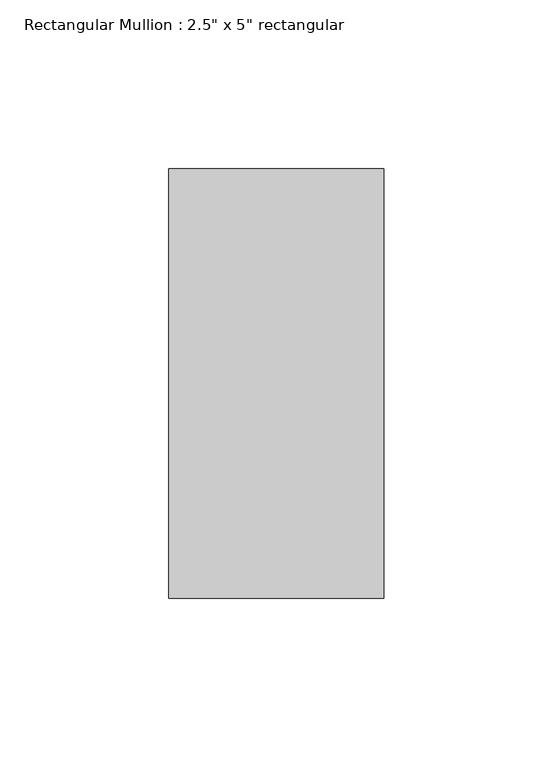
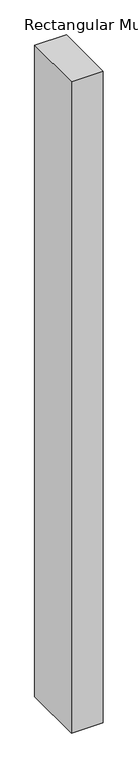
"""IFC4 building model written with IfcOpenShell, lengths in millimetres: member geometry."""

from ifc_helpers import new_model, si_unit, frame, origin, place, context, project, spatial, polyline, outline, extrude, source, transform, mapped, element, save


def member_d76d04ed(model_context):
    return source(origin(), model_context, "Body", "SweptSolid", [
        extrude(outline(polyline([(0.0, 63.5), (0.0, -63.5), (-63.5, -63.5), (-63.5, 63.5), (0.0, 63.5)])), frame((0.0, 0.0, -1376.6336497), z_axis=(0.0, 0.0, 1.0), x_axis=(1.0, 0.0, 0.0)), (0.0, 0.0, 1.0), 1376.6336497),
    ])


if __name__ == "__main__":
    model = new_model("IFC4")
    model_context = context("Model", 3, world=origin())
    ifc_project = project(units=[si_unit("LENGTHUNIT", "METRE", prefix="MILLI")], contexts=[model_context])
    site = spatial("IfcSite", under=ifc_project)
    building = spatial("IfcBuilding", under=site)
    placement = place(None, origin())
    member_shape = member_d76d04ed(model_context)
    element("IfcMember", 1, ObjectType="Rectangular Mullion : 2.5\" x 5\" rectangular", at=placement, inside=building, context=model_context, shape_type="MappedRepresentation", body=[
        mapped(member_shape, transform((0.0, 0.0, 0.0), x_axis=(1.0, 0.0, 0.0), y_axis=(0.0, 1.0, 0.0), z_axis=(0.0, 0.0, 1.0))),
    ])
    save(model, "model.ifc")

# Revit data of these elements
# Type "Rectangular Mullion : 2.5\" x 5\" rectangular"
#   built-in parameter 1007304 = 0.416667 (stored number, unit not read)
#   built-in parameter 1007301 = 0.104167 (stored number, unit not read)
#   built-in parameter 1007300 = 0.104167 (stored number, unit not read)
# Element 1 (IfcMember, "Rectangular Mullion : 2.5\" x 5\" rectangular")
#   Materials on its faces: "Aluminum"
# Materials
#   "Aluminum": class "Metal", colour RGB 247 247 247, transparency 0, Description = "Aluminum 6061", Cost = 0
